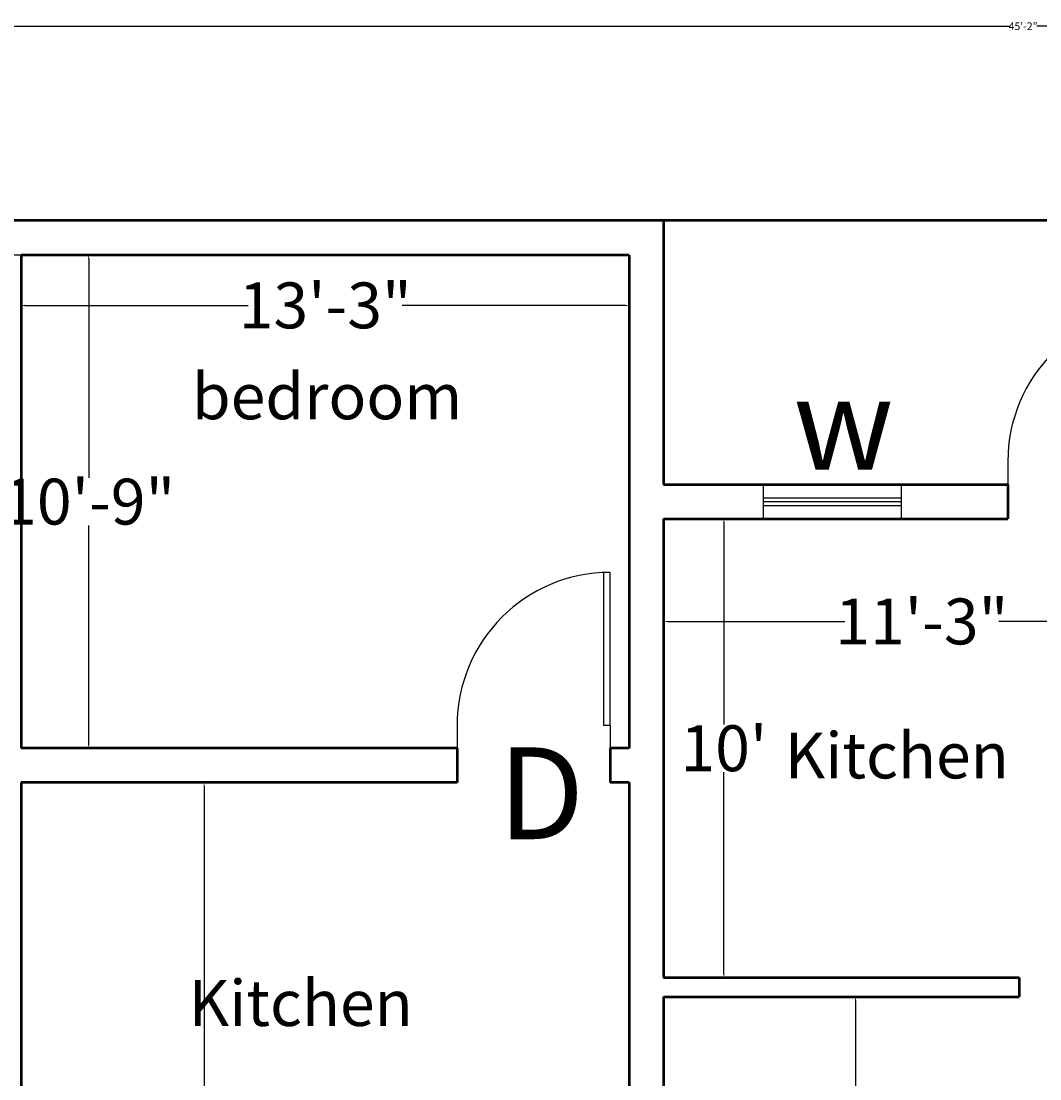
# Model space of a CAD drawing. Units: inches. Extents: x 409 to 7572, y 7 to 725.
# Tile 4 of 38: x 593 to 860, y 448 to 725. Entities that reach past the tile are written whole.
import ezdxf

# ---------------------------------------------------------------- set-up
doc = ezdxf.new("R2010")
doc.units = ezdxf.units.IN
doc.header["$MEASUREMENT"] = 0
for name, color, linetype, lineweight in [('A-ANNO-DIMS', 2, 'Continuous', 18), ('A-ANNO-SYMB', 3, 'Continuous', 25), ('A-AREA-IDEN', 7, 'Continuous', 25), ('A-DOOR', 3, 'Continuous', 25), ('A-GLAZ', 4, 'Continuous', 25), ('A-WALL', 7, 'Continuous', 50)]:
    doc.layers.add(name, color=color, linetype=linetype, lineweight=lineweight)
doc.styles.get("Standard").update_dxf_attribs({"font": 'arial.ttf'})
doc.dimstyles.get("Standard").update_dxf_attribs({"dimtxt": 2, "dimasz": 1, "dimexe": 0.18, "dimexo": 0.0625, "dimgap": 0.09, "dimtad": 0, "dimtih": 1, "dimtoh": 1, "dimdec": 0, "dimzin": 0, "dimdsep": 46, "dimlunit": 3, "dimtxsty": 'Standard', "dimcen": 0.09, "dimadec": 0, "dimazin": 0, "dimtfac": 1, "dimtdec": 0, "dimtofl": 0, "dimtmove": 0, "dimatfit": 3, "dimfxl": 1, "dimtolj": 1, "dimtzin": 0, "dimarcsym": 0})

# ---------------------------------------------------------------- blocks, each defined once
blk = doc.blocks.new('*U2')
for p, q in [((0, 0), (0, -6)), ((-40, 0), (-40, -6))]:
    blk.add_line(p, q)
blk.add_lwpolyline([(0, 0), (0, 40), (-1.75, 40), (-1.75, 0)], close=True)
blk.add_arc((0, 0), 40, 90, 180)
blk = doc.blocks.new('*D9')
at = {"layer": 'A-ANNO-DIMS', "color": 0, "lineweight": -2, "transparency": 16777216}
for p, q in [((593.22, 663.53), (610.99, 663.53)), ((610.81, 662.53), (610.81, 605.25)), ((610.81, 535.53), (610.81, 592.81)), ((593.22, 534.53), (610.99, 534.53))]:
    blk.add_line(p, q, dxfattribs=at)
at = {"layer": 'A-ANNO-DIMS', "color": 0, "transparency": 16777216}
for points in [[(610.64, 662.53), (610.98, 662.53), (610.81, 663.53)], [(610.64, 535.53), (610.98, 535.53), (610.81, 534.53)]]:
    blk.add_solid(points, dxfattribs=at)
at = {"layer": 'DEFPOINTS', "color": 0, "transparency": 16777216}
for p in [(593.16, 663.53), (593.16, 534.53), (610.81, 534.53)]:
    blk.add_point(p, dxfattribs=at)
at = {"layer": 'A-ANNO-DIMS', "color": 0, "transparency": 16777216, "insert": (610.81, 599.03), "char_height": 2, "attachment_point": 5}
blk.add_mtext('\\A1;{\\H6x;10\'-9"}', dxfattribs=at)
blk = doc.blocks.new('*D10')
at = {"layer": 'A-ANNO-DIMS', "color": 0, "lineweight": -2, "transparency": 16777216}
for p, q in [((593.16, 663.47), (593.16, 650.17)), ((752.16, 663.47), (752.16, 650.17)), ((594.16, 650.35), (652.52, 650.35)), ((751.16, 650.35), (692.79, 650.35))]:
    blk.add_line(p, q, dxfattribs=at)
at = {"layer": 'A-ANNO-DIMS', "color": 0, "transparency": 16777216}
for points in [[(594.16, 650.52), (594.16, 650.19), (593.16, 650.35)], [(751.16, 650.52), (751.16, 650.19), (752.16, 650.35)]]:
    blk.add_solid(points, dxfattribs=at)
at = {"layer": 'DEFPOINTS', "color": 0, "transparency": 16777216}
for p in [(593.16, 663.53), (752.16, 663.53), (752.16, 650.35)]:
    blk.add_point(p, dxfattribs=at)
at = {"layer": 'A-ANNO-DIMS', "color": 0, "transparency": 16777216, "insert": (672.66, 650.35), "char_height": 2, "attachment_point": 5}
blk.add_mtext('\\A1;{\\H6x;13\'-3"}', dxfattribs=at)
blk = doc.blocks.new('*D19')
at = {"layer": 'A-ANNO-DIMS', "color": 0, "lineweight": -2, "transparency": 16777216}
for p, q in [((761.22, 594.53), (777.09, 594.53)), ((776.91, 593.53), (776.91, 540.75)), ((776.91, 475.53), (776.91, 528.31)), ((761.22, 474.53), (777.09, 474.53))]:
    blk.add_line(p, q, dxfattribs=at)
at = {"layer": 'A-ANNO-DIMS', "color": 0, "transparency": 16777216}
for points in [[(776.75, 593.53), (777.08, 593.53), (776.91, 594.53)], [(776.75, 475.53), (777.08, 475.53), (776.91, 474.53)]]:
    blk.add_solid(points, dxfattribs=at)
at = {"layer": 'DEFPOINTS', "color": 0, "transparency": 16777216}
for p in [(761.16, 594.53), (761.16, 474.53), (776.91, 474.53)]:
    blk.add_point(p, dxfattribs=at)
at = {"layer": 'A-ANNO-DIMS', "color": 0, "transparency": 16777216, "insert": (776.91, 534.53), "char_height": 2, "attachment_point": 5}
blk.add_mtext("\\A1;{\\H6x;10'}", dxfattribs=at)
blk = doc.blocks.new('*D21')
at = {"layer": 'A-ANNO-DIMS', "color": 0, "lineweight": -2, "transparency": 16777216}
for p, q in [((650.09, 525.53), (640.81, 525.53)), ((640.99, 524.53), (640.99, 428.65)), ((640.99, 320.53), (640.99, 416.42)), ((658.09, 319.53), (640.81, 319.53))]:
    blk.add_line(p, q, dxfattribs=at)
at = {"layer": 'A-ANNO-DIMS', "color": 0, "transparency": 16777216}
for points in [[(640.83, 524.53), (641.16, 524.53), (640.99, 525.53)], [(640.83, 320.53), (641.16, 320.53), (640.99, 319.53)]]:
    blk.add_solid(points, dxfattribs=at)
at = {"layer": 'DEFPOINTS', "color": 0, "transparency": 16777216}
for p in [(650.16, 525.53), (640.99, 319.53), (658.16, 319.53)]:
    blk.add_point(p, dxfattribs=at)
at = {"layer": 'A-ANNO-DIMS', "color": 0, "transparency": 16777216, "insert": (640.99, 422.53), "char_height": 2, "attachment_point": 5}
blk.add_mtext('\\A1;{\\H6x;17\'-2"}', dxfattribs=at)
blk = doc.blocks.new('*D22')
at = {"layer": 'A-ANNO-DIMS', "color": 0, "lineweight": -2, "transparency": 16777216}
for p, q in [((761.16, 563.4), (761.16, 567.87)), ((762.16, 567.69), (808.52, 567.69)), ((895.16, 567.69), (848.79, 567.69)), ((896.16, 563.4), (896.16, 567.87))]:
    blk.add_line(p, q, dxfattribs=at)
at = {"layer": 'A-ANNO-DIMS', "color": 0, "transparency": 16777216}
for points in [[(762.16, 567.86), (762.16, 567.52), (761.16, 567.69)], [(895.16, 567.86), (895.16, 567.52), (896.16, 567.69)]]:
    blk.add_solid(points, dxfattribs=at)
at = {"layer": 'DEFPOINTS', "color": 0, "transparency": 16777216}
for p in [(896.16, 567.69), (761.16, 563.33), (896.16, 563.33)]:
    blk.add_point(p, dxfattribs=at)
at = {"layer": 'A-ANNO-DIMS', "color": 0, "transparency": 16777216, "insert": (828.66, 567.69), "char_height": 2, "attachment_point": 5}
blk.add_mtext('\\A1;{\\H6x;11\'-3"}', dxfattribs=at)
blk = doc.blocks.new('*D24')
at = {"layer": 'A-ANNO-DIMS', "color": 0, "lineweight": -2, "transparency": 16777216}
for p, q in [((815.42, 469.53), (811.17, 469.53)), ((811.35, 468.53), (811.35, 409.65)), ((811.35, 338.53), (811.35, 397.42)), ((816.59, 337.53), (811.17, 337.53))]:
    blk.add_line(p, q, dxfattribs=at)
at = {"layer": 'A-ANNO-DIMS', "color": 0, "transparency": 16777216}
for points in [[(811.19, 468.53), (811.52, 468.53), (811.35, 469.53)], [(811.19, 338.53), (811.52, 338.53), (811.35, 337.53)]]:
    blk.add_solid(points, dxfattribs=at)
at = {"layer": 'DEFPOINTS', "color": 0, "transparency": 16777216}
for p in [(815.48, 469.53), (811.35, 337.53), (816.66, 337.53)]:
    blk.add_point(p, dxfattribs=at)
at = {"layer": 'A-ANNO-DIMS', "color": 0, "transparency": 16777216, "insert": (811.35, 403.53), "char_height": 2, "attachment_point": 5}
blk.add_mtext("\\A1;{\\H6x;11'}", dxfattribs=at)
blk = doc.blocks.new('*D30')
at = {"layer": 'A-ANNO-DIMS', "color": 0, "lineweight": -2, "transparency": 16777216}
for p, q in [((584.16, 672.59), (584.16, 723.56)), ((585.16, 723.38), (851.59, 723.38)), ((1125.16, 723.38), (858.72, 723.38)), ((1126.16, 672.59), (1126.16, 723.56))]:
    blk.add_line(p, q, dxfattribs=at)
at = {"layer": 'A-ANNO-DIMS', "color": 0, "transparency": 16777216}
for points in [[(585.16, 723.55), (585.16, 723.22), (584.16, 723.38)], [(1125.16, 723.55), (1125.16, 723.22), (1126.16, 723.38)]]:
    blk.add_solid(points, dxfattribs=at)
at = {"layer": 'DEFPOINTS', "color": 0, "transparency": 16777216}
for p in [(584.16, 723.38), (584.16, 672.53), (1126.16, 672.53)]:
    blk.add_point(p, dxfattribs=at)
at = {"layer": 'A-ANNO-DIMS', "color": 0, "transparency": 16777216, "insert": (855.16, 723.38), "char_height": 2, "attachment_point": 5}
blk.add_mtext('\\A1;45\'-2"', dxfattribs=at)
blk = doc.blocks.new('WIN-36')
for p, q in [((1699.82, 514.65), (1699.82, 478.65)), ((1700.82, 514.65), (1700.82, 478.65)), ((1701.82, 514.65), (1701.82, 478.65))]:
    blk.add_line(p, q)
blk.add_lwpolyline([(1705.32, 514.65), (1705.32, 478.65), (1696.32, 478.65), (1696.32, 514.65)], close=True)
blk = doc.blocks.new('*D173')
at = {"layer": 'A-ANNO-DIMS', "color": 0, "lineweight": -2, "transparency": 16777216}
for p, q in [((584.09, 672.53), (496.98, 672.53)), ((497.16, 671.53), (497.16, 669.14)), ((497.16, 664.53), (497.16, 666.92)), ((593.09, 663.53), (496.98, 663.53))]:
    blk.add_line(p, q, dxfattribs=at)
at = {"layer": 'A-ANNO-DIMS', "color": 0, "transparency": 16777216}
for points in [[(496.99, 671.53), (497.32, 671.53), (497.16, 672.53)], [(496.99, 664.53), (497.32, 664.53), (497.16, 663.53)]]:
    blk.add_solid(points, dxfattribs=at)
at = {"layer": 'DEFPOINTS', "color": 0, "transparency": 16777216}
for p in [(584.16, 672.53), (497.16, 663.53), (593.16, 663.53)]:
    blk.add_point(p, dxfattribs=at)
at = {"layer": 'A-ANNO-DIMS', "color": 0, "transparency": 16777216, "insert": (497.16, 668.03), "char_height": 2, "attachment_point": 5}
blk.add_mtext('\\A1;0\'-9"', dxfattribs=at)

msp = doc.modelspace()

# ---------------------------------------------------------------- linework, layer by layer
at = {"layer": 'A-WALL'}
for p, q in [((1126.16, 672.53), (584.16, 672.53)), ((761.16, 672.53), (761.16, 603.53)), ((593.16, 663.53), (593.16, 534.53)), ((752.16, 663.53), (593.16, 663.53)), ((752.16, 663.53), (752.16, 534.53)), ((752.16, 663.53), (752.16, 534.53)), ((761.16, 603.53), (851.16, 603.53)), ((851.16, 603.53), (851.16, 594.53)), ((761.16, 594.53), (851.16, 594.53)), ((761.16, 594.53), (761.16, 474.53)), ((707.16, 534.53), (593.16, 534.53)), ((707.16, 534.53), (707.16, 525.53)), ((752.16, 534.53), (747.16, 534.53)), ((747.16, 534.53), (747.16, 525.53)), ((593.16, 525.53), (593.16, 404.53)), ((707.16, 525.53), (593.16, 525.53)), ((752.16, 525.53), (747.16, 525.53)), ((752.16, 525.53), (752.16, 319.53)), ((761.16, 474.53), (854.16, 474.53)), ((854.16, 474.53), (854.16, 469.53)), ((761.16, 469.53), (854.16, 469.53)), ((761.16, 469.53), (761.16, 337.53))]:
    msp.add_line(p, q, dxfattribs=at)

# ---------------------------------------------------------------- block references
at = {"layer": 'A-DOOR'}
for p in [(891.16, 609.53), (747.16, 540.53)]:
    msp.add_blockref('*U2', p, dxfattribs=at)
at = {"layer": 'A-GLAZ', "rotation": 89.9999999999986}
msp.add_blockref('WIN-36', (1301.9, -1101.79), dxfattribs=at)

# ---------------------------------------------------------------- texts
at = {"layer": 'A-ANNO-SYMB', "char_height": 24, "attachment_point": 1}
for s, width, insert in [('w', 18.2582, (795.06, 631.4)), ('D', 19.1972, (717.88, 534.75))]:
    msp.add_mtext_dynamic_manual_height_columns(s, width=width, gutter_width=1, heights=[0], dxfattribs=dict(at, insert=insert))
at = {"layer": 'A-AREA-IDEN', "char_height": 12, "attachment_point": 1}
for s, width, insert in [('bedroom', 40.9017, (637.82, 632.57)), ('Kitchen ', 61.5504, (792.84, 538.64)), ('Kitchen ', 61.5504, (636.98, 473.89))]:
    msp.add_mtext_dynamic_manual_height_columns(s, width=width, gutter_width=1, heights=[0], dxfattribs=dict(at, insert=insert))

# ---------------------------------------------------------------- dimensions: what is measured, and where the dimension line sits
at = {"layer": 'A-ANNO-DIMS'}
dim = msp.add_linear_dim(base=(584.16, 723.38), p1=(1126.16, 672.53), p2=(584.16, 672.53), dimstyle='Standard', override={"dimclrd": 0, "dimclre": 0, "dimclrt": 0}, dxfattribs=at)
dim.commit()
dim.dimension.update_dxf_attribs({"geometry": '*D30', "text_midpoint": (855.16, 723.38)})
dim = msp.add_linear_dim(base=(497.16, 663.53), p1=(584.16, 672.53), p2=(593.16, 663.53), angle=90, dimstyle='Standard', override={"dimdec": 1, "dimlfac": 1, "dimrnd": 0, "dimzin": 1, "dimdsep": 46, "dimlunit": 4, "dimfrac": 2}, dxfattribs=at)
dim.commit()
dim.dimension.update_dxf_attribs({"geometry": '*D173', "text_midpoint": (497.16, 668.03)})
for base, p1, p2, picture, middle in [((610.81, 534.53), (593.16, 663.53), (593.16, 534.53), '*D9', (610.81, 599.03)), ((776.91, 474.53), (761.16, 594.53), (761.16, 474.53), '*D19', (776.91, 534.53)), ((811.35, 337.53), (815.48, 469.53), (816.66, 337.53), '*D24', (811.35, 403.53))]:
    dim = msp.add_linear_dim(base=base, p1=p1, p2=p2, angle=90, text='{\\H6x;<>}', dimstyle='Standard', override={"dimclrd": 0, "dimclre": 0, "dimclrt": 0}, dxfattribs=at)
    dim.commit()
    dim.dimension.update_dxf_attribs({"geometry": picture, "text_midpoint": middle})
for base, p1, p2, picture, middle in [((752.16, 650.35), (593.16, 663.53), (752.16, 663.53), '*D10', (672.66, 650.35)), ((896.16, 567.69), (761.16, 563.33), (896.16, 563.33), '*D22', (828.66, 567.69))]:
    dim = msp.add_linear_dim(base=base, p1=p1, p2=p2, text='{\\H6x;<>}', dimstyle='Standard', override={"dimclrd": 0, "dimclre": 0, "dimclrt": 0}, dxfattribs=at)
    dim.commit()
    dim.dimension.update_dxf_attribs({"geometry": picture, "text_midpoint": middle})
dim = msp.add_linear_dim(base=(640.99, 319.53), p1=(650.16, 525.53), p2=(658.16, 319.53), angle=90, text='{\\H6x;<>}', dimstyle='Standard', override={"dimclrd": 0, "dimclre": 0, "dimclrt": 0}, dxfattribs=at)
dim.commit()
dim.dimension.update_dxf_attribs({"geometry": '*D21', "text_midpoint": (640.99, 422.53), "dimtype": 160})

doc.saveas('drawing.dxf')
